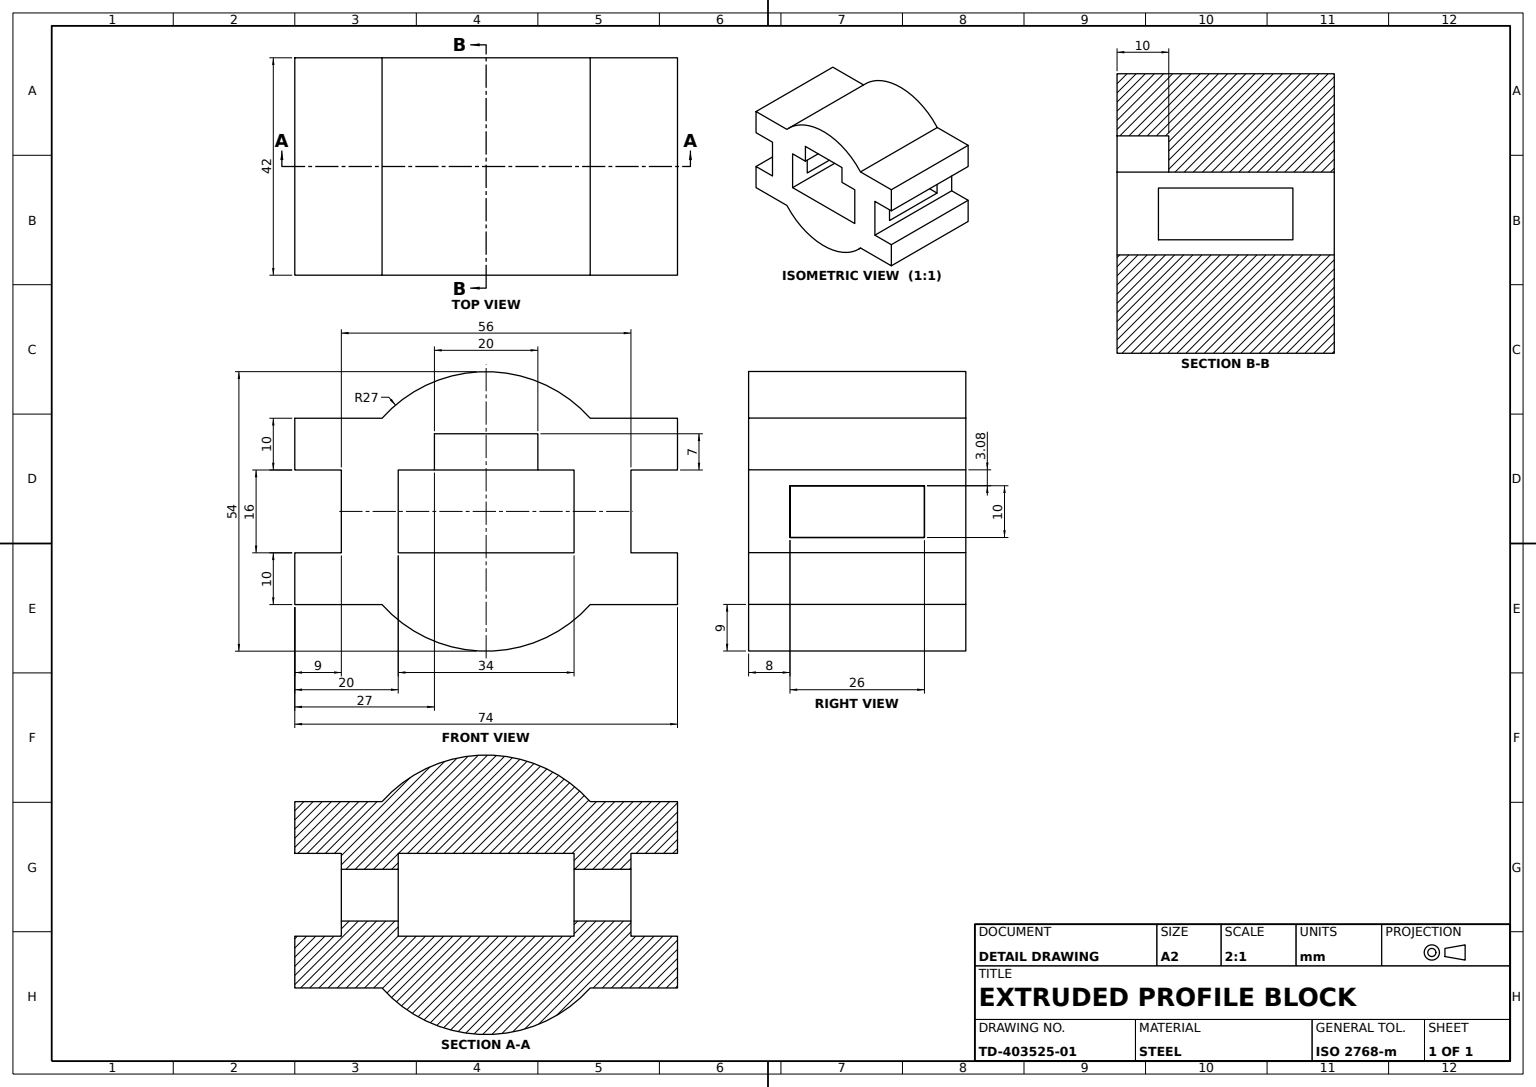
SolidWorks part; units mm, degrees
material "Plain Carbon Steel"
ref_plane "Front Plane" through (0, 0, 0) normal (0, 0, 1) x (1, 0, 0)
ref_plane "Top Plane" through (0, 0, 0) normal (0, 1, 0) x (1, 0, 0)
ref_plane "Right Plane" through (0, 0, 0) normal (1, 0, 0) x (0, 0, -1)
sketch "Block Profile Sketch" plane through (0, 0, 0) normal (0, 0, 1) x (1, 0, 0)
  line L0 (0, 0) -> (16.8754, 0)
  line L1 (74, 0) -> (74, -10)
  line L2 (74, -10) -> (65, -10)
  line L3 (65, -10) -> (65, -26)
  line L4 (65, -26) -> (74, -26)
  line L5 (74, -26) -> (74, -36)
  line L6 (74, -36) -> (57.1246, -36)
  line L7 (57.1246, 0) -> (74, 0)
  line L8 (16.8754, -36) -> (0, -36)
  line L9 (37, -18) -> (37, 9) construction
  line L10 (0, -26) -> (0, -36)
  line L11 (9, -26) -> (0, -26)
  line L12 (9, -10) -> (9, -26)
  line L13 (0, -10) -> (9, -10)
  line L14 (0, 0) -> (0, -10)
  arc A0 (16.8754, -36) -> (57.1246, -36) centre (37, -18) ccw
  arc A1 (57.1246, 0) -> (16.8754, 0) centre (37, -18) ccw
  point P19 (37, -45)
  dimension "D7" = 54
  dimension "D9" = 54
  dimension "D1" = 74
  dimension "D2" = 10
  dimension "D3" = 16
  dimension "D4" = 10
  dimension "D5" = 74
  dimension "D6" = 36
  dimension "D8" = 56
extrude "Block Extrude 42" add sketch "Block Profile Sketch" against normal blind 42
sketch "Through Window Sketch" plane through (0, 0, 0) normal (0, 0, 1) x (1, 0, 0)
  line L2 (47, -10) -> (54, -10)
  line L3 (54, -10) -> (54, -26)
  line L4 (54, -26) -> (20, -26)
  line L5 (20, -26) -> (20, -10)
  line L6 (20, -10) -> (27, -10)
  line L8 (65, -26) -> (65, -10) construction
  line L9 (27, -10) -> (47, -10)
  point P3 (37, -3)
  point P10 (37, -26)
  dimension "D1" = 3
  dimension "D2" = 16
  dimension "D3" = 16
  dimension "D4" = 34
  dimension "D5" = 28
  dimension "D6" = 7
  dimension "D7" = 7
extrude "Through Window Cut" cut sketch "Through Window Sketch" against normal through all
sketch "Pocket 20x7 Sketch" plane through (0, 0, 0) normal (0, 0, 1) x (1, 0, 0)
  line L0 (20, -10) -> (20, -26) construction
  line L1 (54, -10) -> (20, -10) construction
  line L2 (27, -10) -> (27, -3)
  line L3 (27, -3) -> (47, -3)
  line L4 (47, -3) -> (47, -10)
  line L5 (54, -26) -> (54, -10) construction
  line L6 (27, -10) -> (47, -10)
  dimension "D1" = 20
  dimension "D2" = 7
  dimension "D3" = 7
  dimension "D4" = 7
  dimension "D5" = 7
extrude "Pocket 20x7 Depth 10" cut sketch "Pocket 20x7 Sketch" against normal blind 10
sketch "Side Slot Sketch" plane through (9, 0, 0) normal (-1, 0, 0) x (0, 0, 1)
  line L0 (-34, -23.0752) -> (-34, -13.0752)
  line L1 (-34, -13.0752) -> (-8, -13.0752)
  line L2 (-8, -13.0752) -> (-8, -23.0752)
  line L3 (-8, -23.0752) -> (-34, -23.0752)
  line L4 (-42, -10) -> (-42, -26) construction
  line L6 (-42, -10) -> (0, -10) construction
  point P3 (-34, -18.0752)
  dimension "D1" = 26
  dimension "D2" = 10
  dimension "D3" = 8
  dimension "D4" = 3.0752
extrude "Side Slot Cut 26x8" cut sketch "Side Slot Sketch" against normal through all
